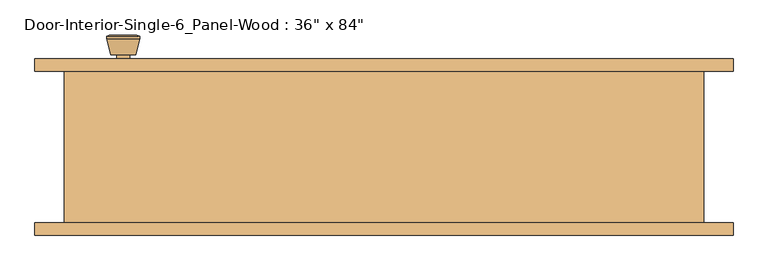
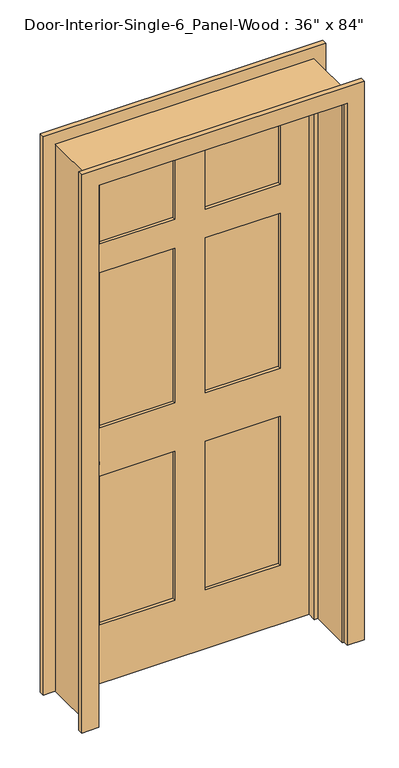
"""IFC4 building model written with IfcOpenShell, lengths in millimetres: door geometry."""

from ifc_helpers import new_model, si_unit, point, frame, frame_2d, origin, place, context, project, spatial, polyline, circle_curve, trimmed, segment, composite_curve, outline, extrude, faceted_brep, source, transform, mapped, element, save
from ifc_brep_helpers import plane_surface, cylinder_surface, revolved_surface, advanced_brep


def door_d86b6c54(model_context):
    return source(origin(), model_context, "Body", "SolidModel", [
        advanced_brep(
        [(-393.7, 70.2, 914.4), (-383.7, 70.2, 914.4), (-403.7, 70.2, 914.4), (-373.2241324, 21.2, 914.4), (-393.7, 21.2, 914.4), (-414.1758676, 21.2, 914.4), (-368.7, 23.0278681, 914.4), (-418.7, 23.0278681, 914.4), (-368.7, 26.4915463, 914.4), (-418.7, 26.4915463, 914.4), (-375.063764, 51.2, 914.4), (-412.336236, 51.2, 914.4), (-383.7, 51.2, 914.4), (-403.7, 51.2, 914.4)],
        [
            (0, 1),
            (1, 2, circle_curve(frame((-393.7, 70.2, 914.4), z_axis=(0.0, 1.0, 0.0), x_axis=(-1.0, 0.0, 0.0)), 10.0)),
            (2, 0),
            (2, 1, circle_curve(frame((-393.7, 70.2, 914.4), z_axis=(0.0, 1.0, 0.0), x_axis=(-1.0, 0.0, 0.0)), 10.0)),
            (3, 4),
            (4, 5),
            (5, 3, circle_curve(frame((-393.7, 21.2, 914.4), z_axis=(0.0, -1.0, 0.0), x_axis=(-1.0, 0.0, 0.0)), 20.4758676)),
            (3, 5, circle_curve(frame((-393.7, 21.2, 914.4), z_axis=(0.0, -1.0, 0.0), x_axis=(-1.0, 0.0, 0.0)), 20.4758676)),
            (6, 3),
            (5, 7),
            (7, 6, circle_curve(frame((-393.7, 23.0278681, 914.4), z_axis=(0.0, -1.0, 0.0), x_axis=(-1.0, 0.0, 0.0)), 25.0)),
            (6, 7, circle_curve(frame((-393.7, 23.0278681, 914.4), z_axis=(0.0, -1.0, 0.0), x_axis=(-1.0, 0.0, 0.0)), 25.0)),
            (8, 6),
            (7, 9),
            (9, 8, circle_curve(frame((-393.7, 26.4915463, 914.4), z_axis=(0.0, -1.0, 0.0), x_axis=(-1.0, 0.0, 0.0)), 25.0)),
            (8, 9, circle_curve(frame((-393.7, 26.4915463, 914.4), z_axis=(0.0, -1.0, 0.0), x_axis=(-1.0, 0.0, 0.0)), 25.0)),
            (10, 8),
            (9, 11),
            (11, 10, circle_curve(frame((-393.7, 51.2, 914.4), z_axis=(0.0, -1.0, 0.0), x_axis=(-1.0, 0.0, 0.0)), 18.636236)),
            (10, 11, circle_curve(frame((-393.7, 51.2, 914.4), z_axis=(0.0, -1.0, 0.0), x_axis=(-1.0, 0.0, 0.0)), 18.636236)),
            (12, 10),
            (11, 13),
            (13, 12, circle_curve(frame((-393.7, 51.2, 914.4), z_axis=(0.0, -1.0, 0.0), x_axis=(-1.0, 0.0, 0.0)), 10.0)),
            (12, 13, circle_curve(frame((-393.7, 51.2, 914.4), z_axis=(0.0, -1.0, 0.0), x_axis=(-1.0, 0.0, 0.0)), 10.0)),
            (1, 12),
            (13, 2),
        ],
        [
            plane_surface(frame((-393.7, 70.2, 914.4), z_axis=(0.0, 1.0, 0.0), x_axis=(-1.0, 0.0, 0.0))),
            plane_surface(frame((-393.7, 21.2, 914.4), z_axis=(0.0, -1.0, 0.0), x_axis=(-1.0, 0.0, 0.0))),
            revolved_surface(polyline([(-414.1758676, 21.2, 914.4), (-418.7, 23.0278681, 914.4)]), (-393.7, 70.2, 914.4), (0.0, 1.0, 0.0)),
            cylinder_surface(frame((-393.7, 70.2, 914.4), z_axis=(0.0, 1.0, 0.0), x_axis=(-1.0, 0.0, 0.0)), 25.0),
            revolved_surface(polyline([(-418.7, 26.4915463, 914.4), (-412.336236, 51.2, 914.4)]), (-393.7, 70.2, 914.4), (0.0, 1.0, 0.0)),
            plane_surface(frame((-393.7, 51.2, 914.4), z_axis=(0.0, 1.0, 0.0), x_axis=(-1.0, 0.0, 0.0))),
            cylinder_surface(frame((-393.7, 70.2, 914.4), z_axis=(0.0, 1.0, 0.0), x_axis=(-1.0, 0.0, 0.0)), 10.0),
        ],
        [
            (0, [[1, 2, 3]]),
            (0, [[-3, 4, -1]]),
            (1, [[5, 6, 7]]),
            (1, [[-6, -5, 8]]),
            (2, [[9, -7, 10, 11]]),
            (2, [[-10, -8, -9, 12]]),
            (3, [[13, -11, 14, 15]]),
            (3, [[-14, -12, -13, 16]]),
            (4, [[17, -15, 18, 19]]),
            (4, [[-18, -16, -17, 20]]),
            (5, [[21, -19, 22, 23]]),
            (5, [[-22, -20, -21, 24]]),
            (6, [[25, -23, 26, -2]]),
            (6, [[-26, -24, -25, -4]]),
        ],
    ),
        extrude(outline(composite_curve([segment(trimmed(circle_curve(frame_2d((914.4, -393.7)), 30.0), [point((914.4, -423.7))], [point((914.4, -363.7))], False, "CARTESIAN"), True, "CONTINUOUS"), segment(trimmed(circle_curve(frame_2d((914.4, -393.7)), 30.0), [point((914.4, -363.7))], [point((914.4, -423.7))], False, "CARTESIAN"), True, "CONTINUOUS")], self_intersect=False)), frame((0.0, 70.2, 0.0), z_axis=(0.0, 1.0, 0.0), x_axis=(0.0, 0.0, 1.0)), (0.0, 0.0, 1.0), 6.0),
        advanced_brep(
        [(-393.7, 117.125, 914.4), (-403.7, 117.125, 914.4), (-383.7, 117.125, 914.4), (-373.2241324, 166.125, 914.4), (-414.1758676, 166.125, 914.4), (-393.7, 166.125, 914.4), (-368.7, 164.2971319, 914.4), (-418.7, 164.2971319, 914.4), (-368.7, 160.8334537, 914.4), (-418.7, 160.8334537, 914.4), (-375.063764, 136.125, 914.4), (-412.336236, 136.125, 914.4), (-383.7, 136.125, 914.4), (-403.7, 136.125, 914.4)],
        [
            (0, 1),
            (1, 2, circle_curve(frame((-393.7, 117.125, 914.4), z_axis=(0.0, -1.0, 0.0), x_axis=(-1.0, 0.0, 0.0)), 10.0)),
            (2, 0),
            (2, 1, circle_curve(frame((-393.7, 117.125, 914.4), z_axis=(0.0, -1.0, 0.0), x_axis=(-1.0, 0.0, 0.0)), 10.0)),
            (3, 4, circle_curve(frame((-393.7, 166.125, 914.4), z_axis=(0.0, 1.0, 0.0), x_axis=(-1.0, 0.0, 0.0)), 20.4758676)),
            (4, 5),
            (5, 3),
            (4, 3, circle_curve(frame((-393.7, 166.125, 914.4), z_axis=(0.0, 1.0, 0.0), x_axis=(-1.0, 0.0, 0.0)), 20.4758676)),
            (6, 7, circle_curve(frame((-393.7, 164.2971319, 914.4), z_axis=(0.0, 1.0, 0.0), x_axis=(-1.0, 0.0, 0.0)), 25.0)),
            (7, 4),
            (3, 6),
            (7, 6, circle_curve(frame((-393.7, 164.2971319, 914.4), z_axis=(0.0, 1.0, 0.0), x_axis=(-1.0, 0.0, 0.0)), 25.0)),
            (8, 9, circle_curve(frame((-393.7, 160.8334537, 914.4), z_axis=(0.0, 1.0, 0.0), x_axis=(-1.0, 0.0, 0.0)), 25.0)),
            (9, 7),
            (6, 8),
            (9, 8, circle_curve(frame((-393.7, 160.8334537, 914.4), z_axis=(0.0, 1.0, 0.0), x_axis=(-1.0, 0.0, 0.0)), 25.0)),
            (10, 11, circle_curve(frame((-393.7, 136.125, 914.4), z_axis=(0.0, 1.0, 0.0), x_axis=(-1.0, 0.0, 0.0)), 18.636236)),
            (11, 9),
            (8, 10),
            (11, 10, circle_curve(frame((-393.7, 136.125, 914.4), z_axis=(0.0, 1.0, 0.0), x_axis=(-1.0, 0.0, 0.0)), 18.636236)),
            (12, 13, circle_curve(frame((-393.7, 136.125, 914.4), z_axis=(0.0, 1.0, 0.0), x_axis=(-1.0, 0.0, 0.0)), 10.0)),
            (13, 11),
            (10, 12),
            (13, 12, circle_curve(frame((-393.7, 136.125, 914.4), z_axis=(0.0, 1.0, 0.0), x_axis=(-1.0, 0.0, 0.0)), 10.0)),
            (1, 13),
            (12, 2),
        ],
        [
            plane_surface(frame((-393.7, 117.125, 914.4), z_axis=(0.0, -1.0, 0.0), x_axis=(-1.0, 0.0, 0.0))),
            plane_surface(frame((-393.7, 166.125, 914.4), z_axis=(0.0, 1.0, 0.0), x_axis=(-1.0, 0.0, 0.0))),
            revolved_surface(polyline([(-414.1758676, 166.125, 914.4), (-418.7, 164.2971319, 914.4)]), (-393.7, 117.125, 914.4), (0.0, -1.0, 0.0)),
            cylinder_surface(frame((-393.7, 117.125, 914.4), z_axis=(0.0, -1.0, 0.0), x_axis=(-1.0, 0.0, 0.0)), 25.0),
            revolved_surface(polyline([(-418.7, 160.8334537, 914.4), (-412.336236, 136.125, 914.4)]), (-393.7, 117.125, 914.4), (0.0, -1.0, 0.0)),
            plane_surface(frame((-393.7, 136.125, 914.4), z_axis=(0.0, -1.0, 0.0), x_axis=(-1.0, 0.0, 0.0))),
            cylinder_surface(frame((-393.7, 117.125, 914.4), z_axis=(0.0, -1.0, 0.0), x_axis=(-1.0, 0.0, 0.0)), 10.0),
        ],
        [
            (0, [[1, 2, 3]]),
            (0, [[-3, 4, -1]]),
            (1, [[5, 6, 7]]),
            (1, [[8, -7, -6]]),
            (2, [[9, 10, -5, 11]]),
            (2, [[12, -11, -8, -10]]),
            (3, [[13, 14, -9, 15]]),
            (3, [[16, -15, -12, -14]]),
            (4, [[17, 18, -13, 19]]),
            (4, [[20, -19, -16, -18]]),
            (5, [[21, 22, -17, 23]]),
            (5, [[24, -23, -20, -22]]),
            (6, [[-2, 25, -21, 26]]),
            (6, [[-4, -26, -24, -25]]),
        ],
    ),
        extrude(outline(composite_curve([segment(trimmed(circle_curve(frame_2d((914.4, -393.7)), 30.0), [point((914.4, -423.7))], [point((914.4, -363.7))], False, "CARTESIAN"), True, "CONTINUOUS"), segment(trimmed(circle_curve(frame_2d((914.4, -393.7)), 30.0), [point((914.4, -363.7))], [point((914.4, -423.7))], False, "CARTESIAN"), True, "CONTINUOUS")], self_intersect=False)), frame((0.0, 111.125, 0.0), z_axis=(0.0, 1.0, 0.0), x_axis=(0.0, 0.0, 1.0)), (0.0, 0.0, 1.0), 6.0),
        faceted_brep([(482.6, 111.125, 0.0), (482.6, -117.475, 0.0), (457.2, -117.475, 0.0), (457.2, 41.275, 0.0), (444.5, 41.275, 0.0), (444.5, 76.2, 0.0), (457.2, 76.2, 0.0), (457.2, 111.125, 0.0), (482.6, 111.125, 2159.0), (482.6, -117.475, 2159.0), (-482.6, -117.475, 2159.0), (-482.6, -117.475, 0.0), (-457.2, -117.475, 0.0), (-457.2, -117.475, 2133.6), (457.2, -117.475, 2133.6), (457.2, 41.275, 2133.6), (-457.2, 41.275, 2133.6), (-457.2, 41.275, 0.0), (-444.5, 41.275, 0.0), (-444.5, 41.275, 2120.9), (444.5, 41.275, 2120.9), (444.5, 76.2, 2120.9), (-444.5, 76.2, 2120.9), (-444.5, 76.2, 0.0), (-457.2, 76.2, 0.0), (-457.2, 76.2, 2133.6), (457.2, 76.2, 2133.6), (457.2, 111.125, 2133.6), (-457.2, 111.125, 2133.6), (-457.2, 111.125, 0.0), (-482.6, 111.125, 0.0), (-482.6, 111.125, 2159.0)], [[[0, 1, 2, 3, 4, 5, 6, 7]], [[1, 0, 8, 9]], [[2, 1, 9, 10, 11, 12, 13, 14]], [[3, 2, 14, 15]], [[4, 3, 15, 16, 17, 18, 19, 20]], [[5, 4, 20, 21]], [[6, 5, 21, 22, 23, 24, 25, 26]], [[7, 6, 26, 27]], [[0, 7, 27, 28, 29, 30, 31, 8]], [[9, 8, 31, 10]], [[15, 14, 13, 16]], [[21, 20, 19, 22]], [[27, 26, 25, 28]], [[30, 29, 24, 23, 18, 17, 12, 11]], [[10, 31, 30, 11]], [[16, 13, 12, 17]], [[22, 19, 18, 23]], [[28, 25, 24, 29]]]),
        extrude(outline(polyline([(2133.6, -457.2), (0.0, -457.2), (0.0, 457.2), (2133.6, 457.2), (2133.6, -457.2)]), holes=[polyline([(2014.5375, 57.15), (2014.5375, 336.55), (1735.1375, 336.55), (1735.1375, 57.15), (2014.5375, 57.15)]), polyline([(1620.8375, 336.55), (1009.65, 336.55), (1009.65, 57.15), (1620.8375, 57.15), (1620.8375, 336.55)]), polyline([(1009.65, -57.15), (1009.65, -336.55), (1620.8375, -336.55), (1620.8375, -57.15), (1009.65, -57.15)]), polyline([(1735.1375, -336.55), (2014.5375, -336.55), (2014.5375, -57.15), (1735.1375, -57.15), (1735.1375, -336.55)]), polyline([(819.15, 57.15), (819.15, 336.55), (231.775, 336.55), (231.775, 57.15), (819.15, 57.15)]), polyline([(231.775, -57.15), (231.775, -336.55), (819.15, -336.55), (819.15, -57.15), (231.775, -57.15)])]), frame((0.0, 76.2, 0.0), z_axis=(0.0, 1.0, 0.0), x_axis=(0.0, 0.0, 1.0)), (0.0, 0.0, 1.0), 34.925),
        extrude(outline(polyline([(336.55, 87.8416667), (57.15, 87.8416667), (57.15, 99.4833333), (336.55, 99.4833333), (336.55, 87.8416667)])), frame((0.0, 0.0, 1735.1375), z_axis=(0.0, 0.0, 1.0), x_axis=(1.0, 0.0, 0.0)), (0.0, 0.0, 1.0), 279.4),
        extrude(outline(polyline([(336.55, 87.8416667), (57.15, 87.8416667), (57.15, 99.4833333), (336.55, 99.4833333), (336.55, 87.8416667)])), frame((0.0, 0.0, 1009.65), z_axis=(0.0, 0.0, 1.0), x_axis=(1.0, 0.0, 0.0)), (0.0, 0.0, 1.0), 611.1875),
        extrude(outline(polyline([(-57.15, 87.8416667), (-336.55, 87.8416667), (-336.55, 99.4833333), (-57.15, 99.4833333), (-57.15, 87.8416667)])), frame((0.0, 0.0, 1009.65), z_axis=(0.0, 0.0, 1.0), x_axis=(1.0, 0.0, 0.0)), (0.0, 0.0, 1.0), 611.1875),
        extrude(outline(polyline([(-57.15, 87.8416667), (-336.55, 87.8416667), (-336.55, 99.4833333), (-57.15, 99.4833333), (-57.15, 87.8416667)])), frame((0.0, 0.0, 1735.1375), z_axis=(0.0, 0.0, 1.0), x_axis=(1.0, 0.0, 0.0)), (0.0, 0.0, 1.0), 279.4),
        extrude(outline(polyline([(336.55, 87.8416667), (57.15, 87.8416667), (57.15, 99.4833333), (336.55, 99.4833333), (336.55, 87.8416667)])), frame((0.0, 0.0, 231.775), z_axis=(0.0, 0.0, 1.0), x_axis=(1.0, 0.0, 0.0)), (0.0, 0.0, 1.0), 587.375),
        extrude(outline(polyline([(-57.15, 87.8416667), (-336.55, 87.8416667), (-336.55, 99.4833333), (-57.15, 99.4833333), (-57.15, 87.8416667)])), frame((0.0, 0.0, 231.775), z_axis=(0.0, 0.0, 1.0), x_axis=(1.0, 0.0, 0.0)), (0.0, 0.0, 1.0), 587.375),
        extrude(outline(polyline([(0.0, 463.55), (0.0, 527.05), (2203.45, 527.05), (2203.45, -527.05), (0.0, -527.05), (0.0, -463.55), (2139.95, -463.55), (2139.95, 463.55), (0.0, 463.55)])), frame((0.0, 111.125, 0.0), z_axis=(0.0, 1.0, 0.0), x_axis=(0.0, 0.0, 1.0)), (0.0, 0.0, 1.0), 19.05),
        extrude(outline(polyline([(0.0, 463.55), (0.0, 527.05), (2203.45, 527.05), (2203.45, -527.05), (0.0, -527.05), (0.0, -463.55), (2139.95, -463.55), (2139.95, 463.55), (0.0, 463.55)])), frame((0.0, -136.525, 0.0), z_axis=(0.0, 1.0, 0.0), x_axis=(0.0, 0.0, 1.0)), (0.0, 0.0, 1.0), 19.05),
    ])


if __name__ == "__main__":
    model = new_model("IFC4")
    model_context = context("Model", 3, world=origin())
    ifc_project = project(units=[si_unit("LENGTHUNIT", "METRE", prefix="MILLI")], contexts=[model_context])
    site = spatial("IfcSite", under=ifc_project)
    building = spatial("IfcBuilding", under=site)
    placement = place(None, origin())
    door_shape = door_d86b6c54(model_context)
    element("IfcDoor", 1, ObjectType="Door-Interior-Single-6_Panel-Wood : 36\" x 84\"", at=placement, inside=building, context=model_context, shape_type="MappedRepresentation", body=[
        mapped(door_shape, transform((0.0, 0.0, 0.0), x_axis=(1.0, 0.0, 0.0), y_axis=(0.0, 1.0, 0.0), z_axis=(0.0, 0.0, 1.0))),
    ])
    save(model, "model.ifc")

# Revit data of these elements
# Type "Door-Interior-Single-6_Panel-Wood : 36\" x 84\""
#   Type Mark = "8"
#   Assembly Code = "C1020300"
#   Analytic Construction = "Wooden"
#   Top Rail = 0' - 4 11/16"
#   Top Panel = 0' - 11"
#   Thickness = 0' - 1 3/8"
#   Thermal Resistance (R) = 2.5876 (h·ft²·°F)/BTU
#   Swing Angle [instance default] = 90.00°
#   Stiles = 0' - 4 3/4"
#   Rough Width = 3' - 2"
#   Rough Height = 7' - 1"
#   Mullion = 0' - 4 1/2"
#   Lock Rail = 0' - 7 1/2"
#   Intermediate Rail = 0' - 4 1/2"
#   Height = 7' - 0"
#   Width = 3' - 0"
#   Heat Transfer Coefficient (U) = 0.3865 BTU/(h·ft²·°F)
#   Bottom Rail = 0' - 9 1/8"
#   Trim Material = Cherry
#   Panel Material = Cherry
#   Frame Material = Cherry
#   Door Handle Material = Aluminum
#   Visual Light Transmittance = 0
#   Solar Heat Gain Coefficient = 0
#   Wall Closure = (empty or 0)
#   Function = (empty or 0)
# Element 1 (IfcDoor, "Door-Interior-Single-6_Panel-Wood : 36\" x 84\"")
#   Materials on its faces: "Cherry", "Aluminum"
# Materials
#   "Cherry": class "Wood", colour RGB 226 177 128, transparency 0, Description = "Prunus Serotina", Cost = 0
#   "Aluminum": class "Metal", colour RGB 247 247 247, transparency 0, Description = "Aluminum 6061", Cost = 0
